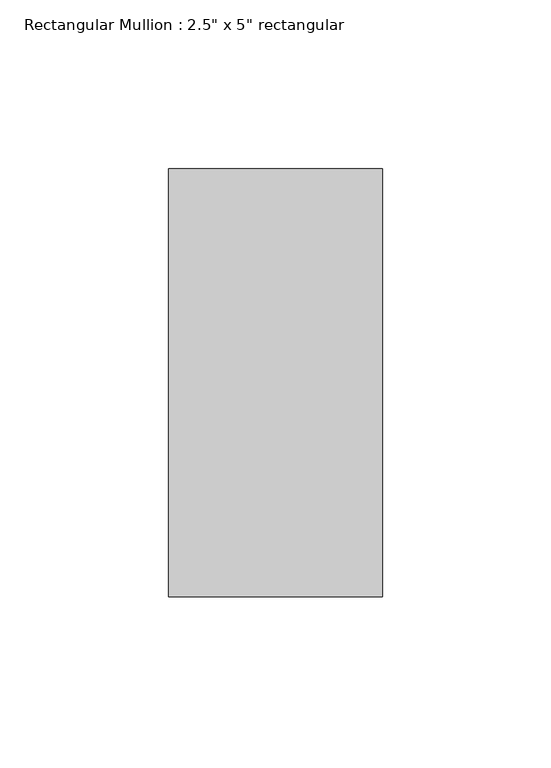
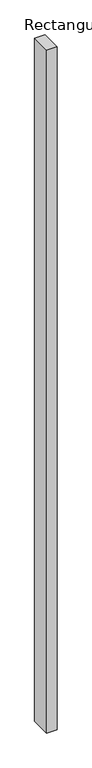
"""IFC4 building model written with IfcOpenShell, lengths in millimetres: member geometry."""

from ifc_helpers import new_model, si_unit, frame, origin, place, context, project, spatial, polyline, outline, extrude, source, transform, mapped, element, save


def member_ad6a65ad(model_context):
    return source(origin(), model_context, "Body", "SweptSolid", [
        extrude(outline(polyline([(0.0, 63.5), (0.0, -63.5), (-63.5, -63.5), (-63.5, 63.5), (0.0, 63.5)])), frame((0.0, 0.0, -4415.4575854), z_axis=(0.0, 0.0, 1.0), x_axis=(1.0, 0.0, 0.0)), (0.0, 0.0, 1.0), 4415.4575854),
    ])


if __name__ == "__main__":
    model = new_model("IFC4")
    model_context = context("Model", 3, world=origin())
    ifc_project = project(units=[si_unit("LENGTHUNIT", "METRE", prefix="MILLI")], contexts=[model_context])
    site = spatial("IfcSite", under=ifc_project)
    building = spatial("IfcBuilding", under=site)
    placement = place(None, origin())
    member_shape = member_ad6a65ad(model_context)
    element("IfcMember", 1, ObjectType="Rectangular Mullion : 2.5\" x 5\" rectangular", at=placement, inside=building, context=model_context, shape_type="MappedRepresentation", body=[
        mapped(member_shape, transform((0.0, 0.0, 0.0), x_axis=(1.0, 0.0, 0.0), y_axis=(0.0, 1.0, 0.0), z_axis=(0.0, 0.0, 1.0))),
    ])
    save(model, "model.ifc")

# Revit data of these elements
# Type "Rectangular Mullion : 2.5\" x 5\" rectangular"
#   built-in parameter 1007304 = 0.416667 (stored number, unit not read)
#   built-in parameter 1007301 = 0.104167 (stored number, unit not read)
#   built-in parameter 1007300 = 0.104167 (stored number, unit not read)
# Element 1 (IfcMember, "Rectangular Mullion : 2.5\" x 5\" rectangular")
#   Materials on its faces: "Aluminum"
# Materials
#   "Aluminum": class "Metal", colour RGB 247 247 247, transparency 0, Description = "Aluminum 6061", Cost = 0
